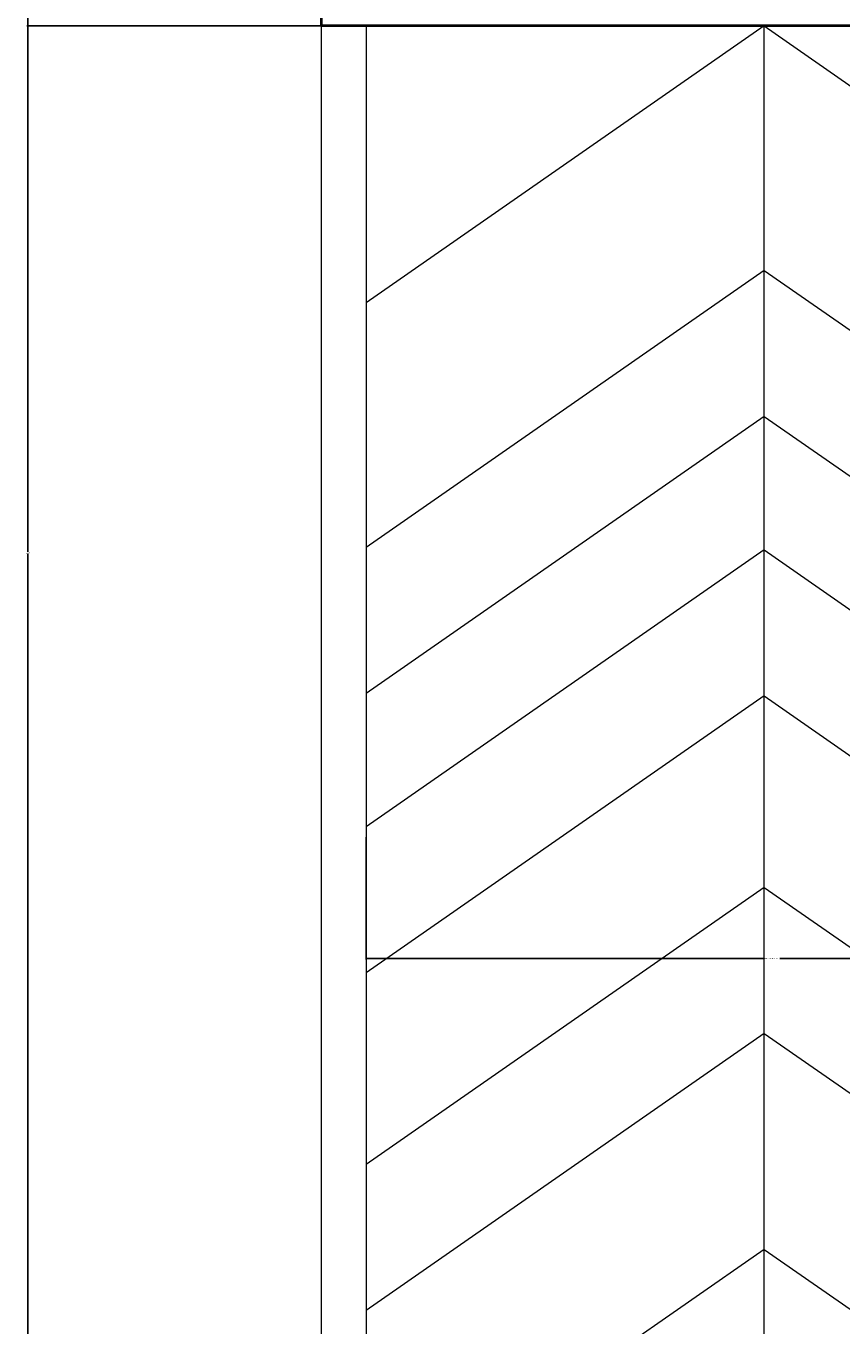
# Model space of a CAD drawing. Units: inches. Extents: x -46 to 1145, y -527 to 760.
# Tile 15 of 57: x -46 to 117, y -38 to 222. Entities that reach past the tile are written whole.
import ezdxf

# ---------------------------------------------------------------- set-up
doc = ezdxf.new("R2010")
doc.units = ezdxf.units.IN
doc.header["$MEASUREMENT"] = 0
for name, color, linetype, lineweight in [('A-ANNO-DIMS', 2, 'Continuous', 18), ('C-ROAD', 9, 'Continuous', 18), ('WALLS', 4, 'Continuous', 40)]:
    doc.layers.add(name, color=color, linetype=linetype, lineweight=lineweight)
doc.styles.get("Standard").update_dxf_attribs({"font": 'arial.ttf'})
doc.dimstyles.get("Standard").update_dxf_attribs({"dimtxt": 0.18, "dimasz": 0.18, "dimexe": 0.18, "dimexo": 0.0625, "dimgap": 0.09, "dimtad": 0, "dimtih": 1, "dimtoh": 1, "dimdec": 0, "dimzin": 0, "dimdsep": 46, "dimlunit": 3, "dimtxsty": 'Standard', "dimcen": 0.09, "dimadec": 0, "dimazin": 0, "dimtfac": 1, "dimtdec": 0, "dimtofl": 0, "dimtmove": 0, "dimatfit": 3, "dimfxl": 1, "dimtolj": 1, "dimtzin": 0, "dimarcsym": 0})

# ---------------------------------------------------------------- blocks, each defined once
blk = doc.blocks.new('DRIVEWAY-CHEVRON')
for q in [(0, 2.03), (162, 0)]:
    blk.add_line((79.54, 57.38), q)
blk = doc.blocks.new('*D656')
at = {"layer": 'A-ANNO-DIMS', "color": 0, "lineweight": -2, "transparency": 16777216}
for p, q in [((21.56, 59.32), (21.56, 34.9)), ((183.56, 59.32), (183.56, 34.9)), ((21.74, 35.08), (100.93, 35.08)), ((183.38, 35.08), (104.2, 35.08))]:
    blk.add_line(p, q, dxfattribs=at)
at = {"layer": 'A-ANNO-DIMS', "color": 0, "transparency": 16777216}
for points in [[(21.74, 35.11), (21.74, 35.05), (21.56, 35.08)], [(183.38, 35.11), (183.38, 35.05), (183.56, 35.08)]]:
    blk.add_solid(points, dxfattribs=at)
at = {"layer": 'Defpoints', "color": 0, "transparency": 16777216}
for p in [(21.56, 59.38), (183.56, 59.38), (183.56, 35.08)]:
    blk.add_point(p, dxfattribs=at)
at = {"layer": 'A-ANNO-DIMS', "color": 0, "transparency": 16777216, "insert": (102.56, 35.08), "char_height": 0.18, "attachment_point": 5}
blk.add_mtext('\\A1;DRIVE MARKING 162 TYP.', dxfattribs=at)
blk = doc.blocks.new('*D685')
at = {"layer": 'A-ANNO-DIMS', "color": 0, "lineweight": -2, "transparency": 16777216}
for p, q in [((183.5, 700.89), (-46.22, 700.89)), ((-46.04, 700.71), (-46.04, 116.39)), ((-46.04, -468.3), (-46.04, 116.02)), ((12.5, -468.48), (-46.22, -468.48))]:
    blk.add_line(p, q, dxfattribs=at)
at = {"layer": 'A-ANNO-DIMS', "color": 0, "transparency": 16777216}
for points in [[(-46.07, 700.71), (-46.01, 700.71), (-46.04, 700.89)], [(-46.07, -468.3), (-46.01, -468.3), (-46.04, -468.48)]]:
    blk.add_solid(points, dxfattribs=at)
at = {"layer": 'Defpoints', "color": 0, "transparency": 16777216}
for p in [(-46.04, 700.89), (183.56, 700.89), (12.56, -468.48)]:
    blk.add_point(p, dxfattribs=at)
at = {"layer": 'A-ANNO-DIMS', "color": 0, "transparency": 16777216, "insert": (-46.04, 116.2), "char_height": 0.18, "attachment_point": 5}
blk.add_mtext('\\A1;1169.4', dxfattribs=at)
blk = doc.blocks.new('*D698')
at = {"layer": 'A-ANNO-DIMS', "color": 0, "lineweight": -2, "transparency": 16777216}
for p, q in [((12.5, 324.33), (-46.22, 324.33)), ((-46.04, 324.15), (-46.04, 273.11)), ((-46.04, 221.7), (-46.04, 272.74)), ((12.5, 221.52), (-46.22, 221.52))]:
    blk.add_line(p, q, dxfattribs=at)
at = {"layer": 'A-ANNO-DIMS', "color": 0, "transparency": 16777216}
for points in [[(-46.07, 324.15), (-46.01, 324.15), (-46.04, 324.33)], [(-46.07, 221.7), (-46.01, 221.7), (-46.04, 221.52)]]:
    blk.add_solid(points, dxfattribs=at)
at = {"layer": 'Defpoints', "color": 0, "transparency": 16777216}
for p in [(-46.04, 324.33), (12.56, 324.33), (12.56, 221.52)]:
    blk.add_point(p, dxfattribs=at)
at = {"layer": 'A-ANNO-DIMS', "color": 0, "transparency": 16777216, "insert": (-46.04, 272.92), "char_height": 0.18, "attachment_point": 5}
blk.add_mtext('\\A1;102.81', dxfattribs=at)

msp = doc.modelspace()

# ---------------------------------------------------------------- linework, layer by layer
at = {"layer": 'C-ROAD'}
for p, q in [((12.5637, 221.5176), (12.5637, -468.4824)), ((21.5637, 221.5176), (21.5637, -459.4824)), ((101.1042, -459.4824), (101.1042, 221.5176))]:
    msp.add_line(p, q, dxfattribs=at)
at = {"layer": 'WALLS'}
for p in [(12.5637, 659.5176), (208.2731, 221.5176)]:
    msp.add_line(p, (12.5637, 221.5176), dxfattribs=at)

# ---------------------------------------------------------------- block references
at = {"layer": 'C-ROAD'}
for p in [(21.564, 164.14), (21.564, 115.245), (21.564, 86.052), (21.564, 59.3801), (21.564, 30.1871), (21.564, -8.1106), (21.564, -37.3036), (21.564, -80.4757)]:
    msp.add_blockref('DRIVEWAY-CHEVRON', p, dxfattribs=at)

# ---------------------------------------------------------------- dimensions: what is measured, and where the dimension line sits
at = {"layer": 'A-ANNO-DIMS'}
for base, p1, p2, override, picture, middle in [((-46.0363, 700.8886), (12.5637, -468.4824), (183.5637, 700.8886), {"dimdec": 1, "dimlfac": 1, "dimrnd": 0, "dimzin": 0, "dimdsep": 46, "dimlunit": 2}, '*D685', (-46.0363, 116.2031)), ((-46.0363, 324.3307), (12.5637, 221.5176), (12.5637, 324.3307), {"dimdec": 2, "dimlfac": 1, "dimrnd": 0, "dimzin": 0, "dimdsep": 46, "dimlunit": 2}, '*D698', (-46.0363, 272.9242))]:
    dim = msp.add_linear_dim(base=base, p1=p1, p2=p2, angle=90, dimstyle='Standard', override=override, dxfattribs=at)
    dim.commit()
    dim.dimension.update_dxf_attribs({"geometry": picture, "text_midpoint": middle})
dim = msp.add_linear_dim(base=(183.5637, 35.0798), p1=(21.5637, 59.3798), p2=(183.5637, 59.3798), text='DRIVE MARKING <> TYP.', dimstyle='Standard', override={"dimdec": 0, "dimlfac": 1, "dimrnd": 0, "dimzin": 0, "dimdsep": 46, "dimlunit": 2}, dxfattribs=at)
dim.commit()
dim.dimension.update_dxf_attribs({"geometry": '*D656', "text_midpoint": (102.5637, 35.0798)})

doc.saveas('drawing.dxf')
